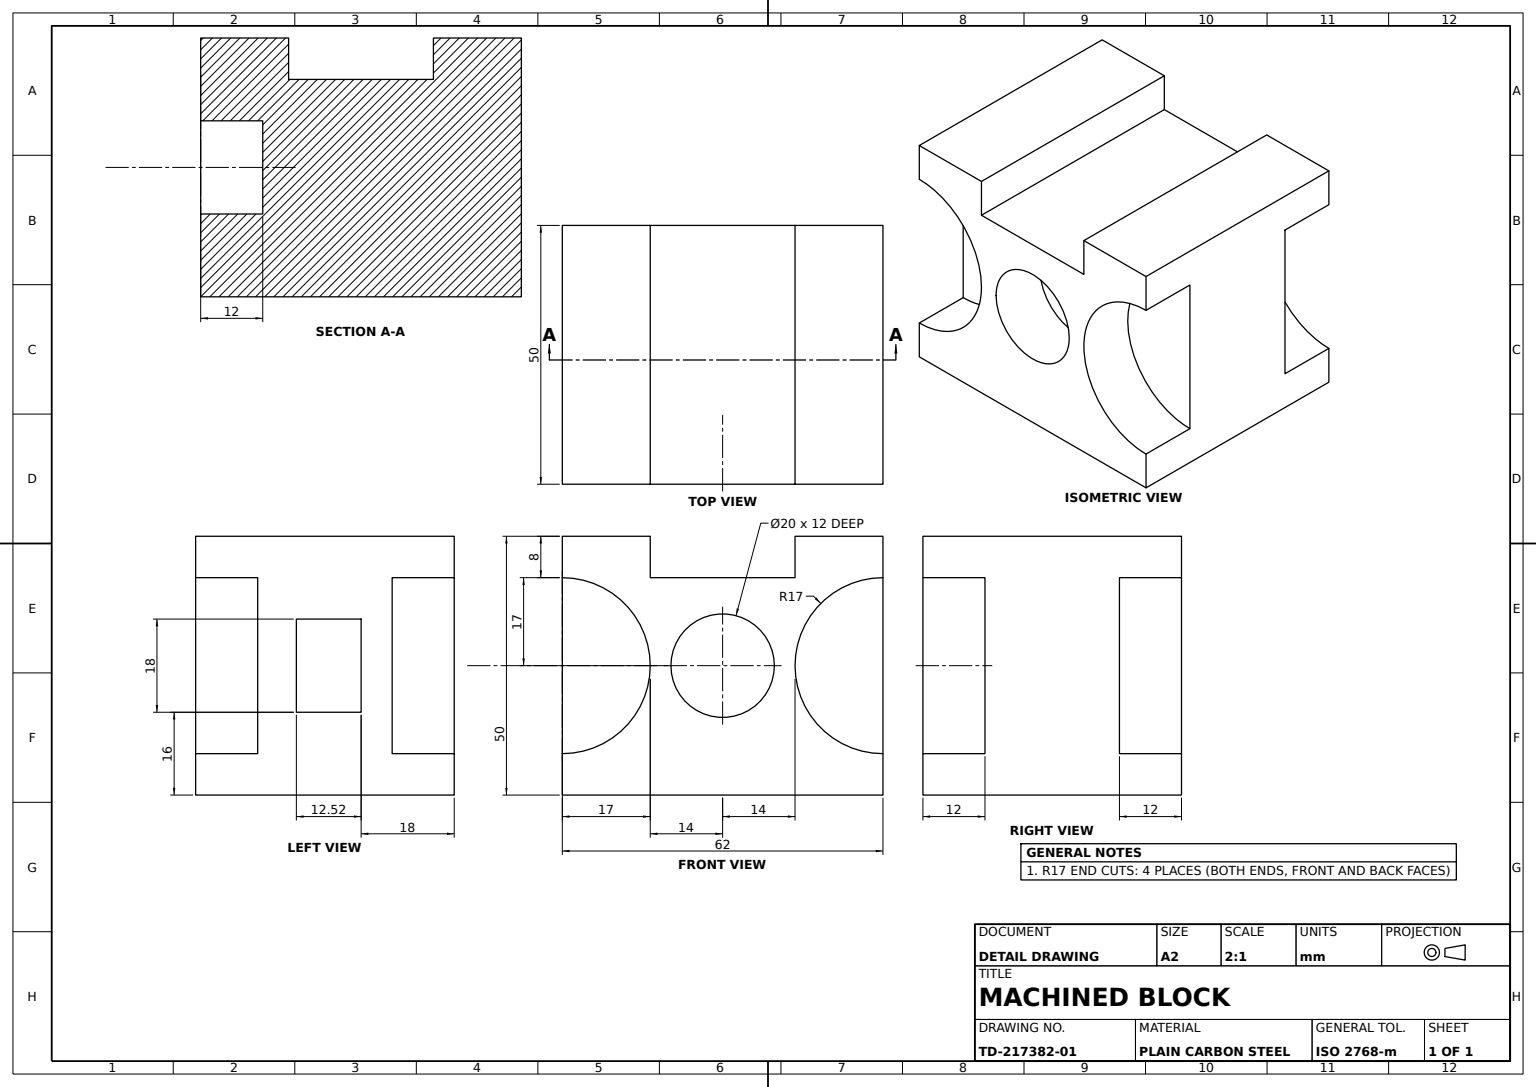
from build123d import *

# Parameters (mm, degrees)
BLOCK_PROFILE_62X50_W             = 62
BLOCK_PROFILE_62X50_H             = 50
BASE_BLOCK_62X50X50_DEPTH         = 50
SQUARE_CUT_A_PROFILE_34X34_R      = 17
SQUARE_CUT_A_34X34_DEPTH_12_DEPTH = 12
SIDE_ARC_CUT_A_DEPTH              = 95.042543564
SIDE_ARC_CUT_B_DEPTH_12_DEPTH     = 12
SQUARE_START                      = -12
SQUARE_CUT_B_PROFILE_34X34_R      = 17
SQUARE_CUT_B_34X34_DEPTH_12_DEPTH = 12
HOLE_PROFILE_20_R                 = 10
HOLE_20_DEPTH_12_DEPTH            = 12


with BuildPart() as part:
    # Block Profile 62x50 → Base Block 62x50x50 (new body)
    with BuildSketch(Plane.XY):
        with Locations((31, 25)):
            Rectangle(BLOCK_PROFILE_62X50_W, BLOCK_PROFILE_62X50_H)
    extrude(amount=BASE_BLOCK_62X50X50_DEPTH)

    # Square Cut A Profile 34x34 → Square Cut A 34x34 Depth 12 (cut)
    with BuildSketch(Plane.XY.offset(50)):
        with Locations((62, 25)):
            Circle(SQUARE_CUT_A_PROFILE_34X34_R)
        with Locations((0, 25)):
            Circle(SQUARE_CUT_A_PROFILE_34X34_R)
    extrude(amount=-SQUARE_CUT_A_34X34_DEPTH_12_DEPTH, mode=Mode.SUBTRACT)

    # Side Arc Cut A Profile → Side Arc Cut A (cut, through all)
    with BuildSketch(Plane.XY.offset(50)):
        Polygon((31, 42), (17, 42), (17, 50), (45, 50), (45, 42), align=None)
    extrude(amount=-SIDE_ARC_CUT_A_DEPTH, mode=Mode.SUBTRACT)

    # Side Arc Cut B Profile → Side Arc Cut B Depth 12 (cut)
    with BuildSketch(Plane.ZY):
        Polygon((25, 34), (19.475936602, 34), (19.475936602, 16), (32, 16), (32, 34), align=None)
    extrude(amount=-SIDE_ARC_CUT_B_DEPTH_12_DEPTH, mode=Mode.SUBTRACT)

    # Square Cut B Profile 34x34 → Square Cut B 34x34 Depth 12 (cut)
    with BuildSketch(Plane(origin=(0, 0, 0), x_dir=(-1, 0, 0), z_dir=(0, 0, -1)).offset(SQUARE_START)):
        with Locations((-62, 25)):
            Circle(SQUARE_CUT_B_PROFILE_34X34_R)
        with Locations((0, 25)):
            Circle(SQUARE_CUT_B_PROFILE_34X34_R)
    extrude(amount=SQUARE_CUT_B_34X34_DEPTH_12_DEPTH, mode=Mode.SUBTRACT)

    # Hole Profile Ø20 → Hole Ø20 Depth 12 (cut)
    with BuildSketch(Plane.XY.offset(50)):
        with Locations((31, 25)):
            Circle(HOLE_PROFILE_20_R)
    extrude(amount=-HOLE_20_DEPTH_12_DEPTH, mode=Mode.SUBTRACT)


solid = part.part
